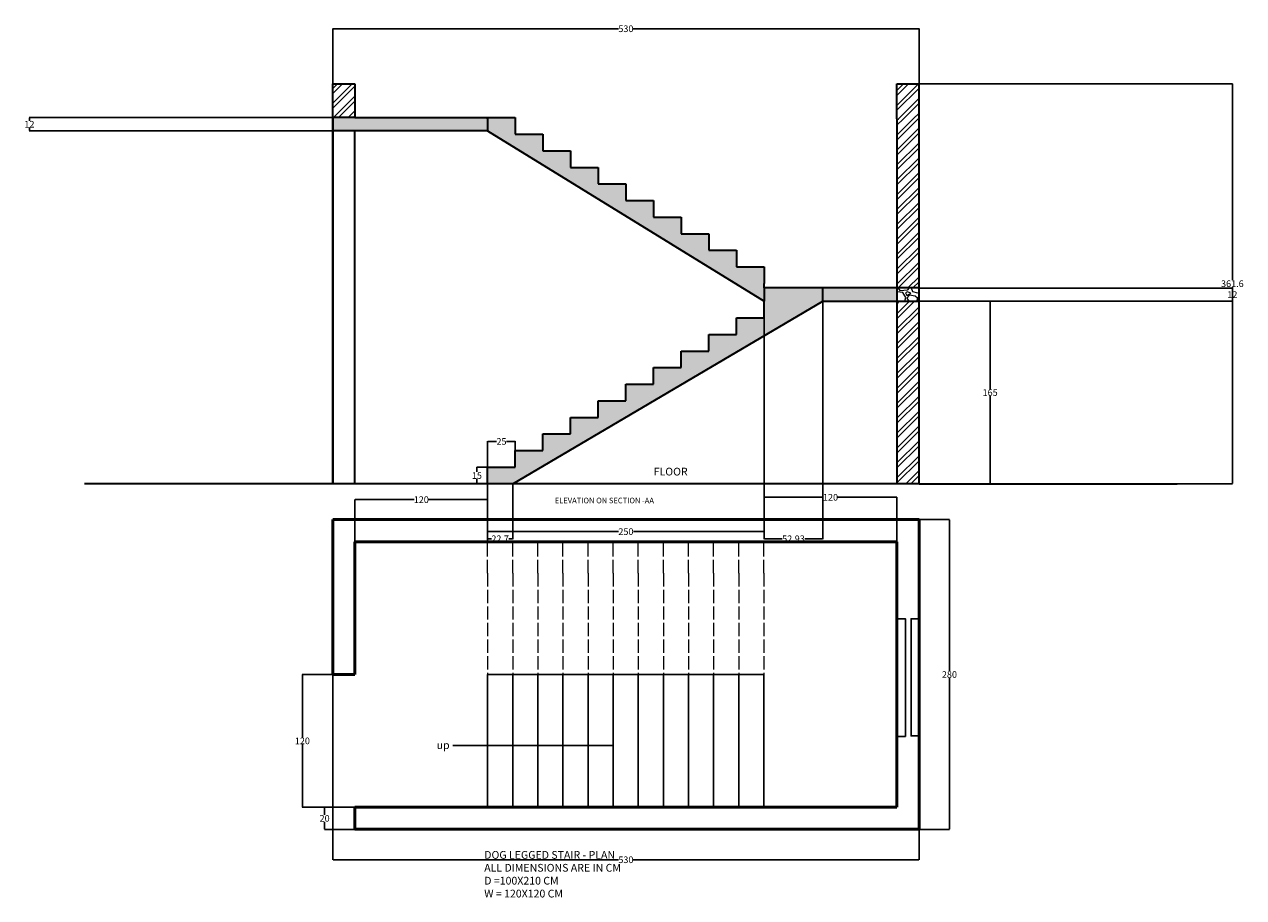
# Model space of a CAD drawing. Units: centimetres. Extents: x 1453 to 2556, y 1176 to 1965.
import ezdxf

# ---------------------------------------------------------------- set-up
doc = ezdxf.new("R2010")
doc.units = ezdxf.units.CM
doc.linetypes.add('ACAD_ISO02W100', pattern=[15, 12, -3])
for name, color, linetype, lineweight in [('A-ANNO-DIMS', 2, 'Continuous', 18), ('A-ANNO-TEXT', 7, 'Continuous', 18), ('A-FLOR-STRS', 3, 'Continuous', 25), ('A-FLOR-STRS-OVHD', 3, 'ACAD_ISO02W100', 18), ('A-GLAZ', 4, 'Continuous', 25), ('A-SECT', 1, 'Continuous', 35), ('A-WALL', 7, 'Continuous', 50), ('A-WALL-PATT', 8, 'Continuous', 18)]:
    doc.layers.add(name, color=color, linetype=linetype, lineweight=lineweight)
doc.styles.get("Standard").update_dxf_attribs({"font": 'arial.ttf'})
doc.dimstyles.get("Standard").update_dxf_attribs({"dimtxt": 6, "dimasz": 0.18, "dimexe": 0.18, "dimexo": 0.0625, "dimgap": 0.09, "dimtad": 0, "dimtih": 1, "dimtoh": 1, "dimdec": 0, "dimzin": 0, "dimdsep": 46, "dimtxsty": 'Standard', "dimcen": 0.09, "dimadec": 0, "dimazin": 0, "dimtfac": 1, "dimtdec": 0, "dimtofl": 0, "dimtmove": 0, "dimatfit": 3, "dimfxl": 1, "dimtolj": 1, "dimtzin": 0, "dimarcsym": 0})

# ---------------------------------------------------------------- blocks, each defined once
blk = doc.blocks.new('*D1')
at = {"layer": 'A-ANNO-DIMS', "color": 0, "lineweight": -2, "transparency": 16777216}
for p, q in [((1752.1, 1257.4), (1724.6, 1257.4)), ((1724.8, 1257.3), (1724.8, 1250.6)), ((1752.1, 1237.4), (1724.6, 1237.4)), ((1724.8, 1237.6), (1724.8, 1244.3))]:
    blk.add_line(p, q, dxfattribs=at)
at = {"layer": 'A-ANNO-DIMS', "color": 0, "transparency": 16777216}
for points in [[(1724.8, 1257.3), (1724.8, 1257.3), (1724.8, 1257.4)], [(1724.8, 1237.6), (1724.8, 1237.6), (1724.8, 1237.4)]]:
    blk.add_solid(points, dxfattribs=at)
at = {"layer": 'Defpoints', "color": 0, "transparency": 16777216}
for p in [(1752.2, 1257.4), (1724.8, 1237.4), (1752.2, 1237.4)]:
    blk.add_point(p, dxfattribs=at)
at = {"layer": 'A-ANNO-DIMS', "color": 0, "transparency": 16777216, "insert": (1724.8, 1247.4), "char_height": 6, "attachment_point": 5}
blk.add_mtext('\\A1;20', dxfattribs=at)
blk = doc.blocks.new('*D2')
at = {"layer": 'A-ANNO-DIMS', "color": 0, "lineweight": -2, "transparency": 16777216}
for p, q in [((1752.2, 1497.5), (1752.2, 1535.7)), ((1752.4, 1535.5), (1805.8, 1535.5)), ((1872, 1535.5), (1818.6, 1535.5)), ((1872.2, 1497.5), (1872.2, 1535.7))]:
    blk.add_line(p, q, dxfattribs=at)
at = {"layer": 'A-ANNO-DIMS', "color": 0, "transparency": 16777216}
for points in [[(1752.4, 1535.5), (1752.4, 1535.5), (1752.2, 1535.5)], [(1872, 1535.5), (1872, 1535.5), (1872.2, 1535.5)]]:
    blk.add_solid(points, dxfattribs=at)
at = {"layer": 'Defpoints', "color": 0, "transparency": 16777216}
for p in [(1752.2, 1535.5), (1752.2, 1497.4), (1872.2, 1497.4)]:
    blk.add_point(p, dxfattribs=at)
at = {"layer": 'A-ANNO-DIMS', "color": 0, "transparency": 16777216, "insert": (1812.2, 1535.5), "char_height": 6, "attachment_point": 5}
blk.add_mtext('\\A1;120', dxfattribs=at)
blk = doc.blocks.new('*D3')
at = {"layer": 'A-ANNO-DIMS', "color": 0, "lineweight": -2, "transparency": 16777216}
for p, q in [((1872.2, 1517.4), (1872.2, 1506.5)), ((2122.2, 1517.4), (2122.2, 1506.5)), ((1872.4, 1506.6), (1990.4, 1506.6)), ((2122, 1506.6), (2004, 1506.6))]:
    blk.add_line(p, q, dxfattribs=at)
at = {"layer": 'A-ANNO-DIMS', "color": 0, "transparency": 16777216}
for points in [[(1872.4, 1506.7), (1872.4, 1506.6), (1872.2, 1506.6)], [(2122, 1506.7), (2122, 1506.6), (2122.2, 1506.6)]]:
    blk.add_solid(points, dxfattribs=at)
at = {"layer": 'Defpoints', "color": 0, "transparency": 16777216}
for p in [(1872.2, 1517.4), (2122.2, 1517.4), (2122.2, 1506.6)]:
    blk.add_point(p, dxfattribs=at)
at = {"layer": 'A-ANNO-DIMS', "color": 0, "transparency": 16777216, "insert": (1997.2, 1506.6), "char_height": 6, "attachment_point": 5}
blk.add_mtext('\\A1;250', dxfattribs=at)
blk = doc.blocks.new('*D4')
at = {"layer": 'A-ANNO-DIMS', "color": 0, "lineweight": -2, "transparency": 16777216}
for p, q in [((2122.2, 1517.5), (2122.2, 1537.7)), ((2122.4, 1537.6), (2175.8, 1537.6)), ((2242, 1537.6), (2188.6, 1537.6)), ((2242.2, 1497.5), (2242.2, 1537.7))]:
    blk.add_line(p, q, dxfattribs=at)
at = {"layer": 'A-ANNO-DIMS', "color": 0, "transparency": 16777216}
for points in [[(2122.4, 1537.6), (2122.4, 1537.5), (2122.2, 1537.6)], [(2242, 1537.6), (2242, 1537.5), (2242.2, 1537.6)]]:
    blk.add_solid(points, dxfattribs=at)
at = {"layer": 'Defpoints', "color": 0, "transparency": 16777216}
for p in [(2242.2, 1537.6), (2122.2, 1517.4), (2242.2, 1497.4)]:
    blk.add_point(p, dxfattribs=at)
at = {"layer": 'A-ANNO-DIMS', "color": 0, "transparency": 16777216, "insert": (2182.2, 1537.6), "char_height": 6, "attachment_point": 5}
blk.add_mtext('\\A1;120', dxfattribs=at)
blk = doc.blocks.new('*D5')
at = {"layer": 'A-ANNO-DIMS', "color": 0, "lineweight": -2, "transparency": 16777216}
for p, q in [((1872.1, 1564.8), (1862.3, 1564.8)), ((1862.5, 1564.7), (1862.5, 1560.5)), ((1872.1, 1549.8), (1862.3, 1549.8)), ((1862.5, 1550), (1862.5, 1554.2))]:
    blk.add_line(p, q, dxfattribs=at)
at = {"layer": 'A-ANNO-DIMS', "color": 0, "transparency": 16777216}
for points in [[(1862.5, 1564.7), (1862.5, 1564.7), (1862.5, 1564.8)], [(1862.5, 1550), (1862.5, 1550), (1862.5, 1549.8)]]:
    blk.add_solid(points, dxfattribs=at)
at = {"layer": 'Defpoints', "color": 0, "transparency": 16777216}
for p in [(1862.5, 1564.8), (1872.2, 1564.8), (1872.2, 1549.8)]:
    blk.add_point(p, dxfattribs=at)
at = {"layer": 'A-ANNO-DIMS', "color": 0, "transparency": 16777216, "insert": (1862.5, 1557.3), "char_height": 6, "attachment_point": 5}
blk.add_mtext('\\A1;15', dxfattribs=at)
blk = doc.blocks.new('*D6')
at = {"layer": 'A-ANNO-DIMS', "color": 0, "lineweight": -2, "transparency": 16777216}
for p, q in [((1872.2, 1564.9), (1872.2, 1588.3)), ((1872.4, 1588.1), (1880.2, 1588.1)), ((1897, 1588.1), (1889.2, 1588.1)), ((1897.2, 1564.9), (1897.2, 1588.3))]:
    blk.add_line(p, q, dxfattribs=at)
at = {"layer": 'A-ANNO-DIMS', "color": 0, "transparency": 16777216}
for points in [[(1872.4, 1588.2), (1872.4, 1588.1), (1872.2, 1588.1)], [(1897, 1588.2), (1897, 1588.1), (1897.2, 1588.1)]]:
    blk.add_solid(points, dxfattribs=at)
at = {"layer": 'Defpoints', "color": 0, "transparency": 16777216}
for p in [(1897.2, 1588.1), (1872.2, 1564.8), (1897.2, 1564.8)]:
    blk.add_point(p, dxfattribs=at)
at = {"layer": 'A-ANNO-DIMS', "color": 0, "transparency": 16777216, "insert": (1884.7, 1588.1), "char_height": 6, "attachment_point": 5}
blk.add_mtext('\\A1;25', dxfattribs=at)
blk = doc.blocks.new('*D7')
at = {"layer": 'A-ANNO-DIMS', "color": 0, "lineweight": -2, "transparency": 16777216}
for p, q in [((2262.3, 1714.8), (2326.7, 1714.8)), ((2326.5, 1714.7), (2326.5, 1635.5)), ((2326.5, 1550), (2326.5, 1629.2)), ((2262.3, 1549.8), (2326.7, 1549.8))]:
    blk.add_line(p, q, dxfattribs=at)
at = {"layer": 'A-ANNO-DIMS', "color": 0, "transparency": 16777216}
for points in [[(2326.5, 1714.7), (2326.6, 1714.7), (2326.5, 1714.8)], [(2326.5, 1550), (2326.6, 1550), (2326.5, 1549.8)]]:
    blk.add_solid(points, dxfattribs=at)
at = {"layer": 'Defpoints', "color": 0, "transparency": 16777216}
for p in [(2262.2, 1714.8), (2326.5, 1714.8), (2262.2, 1549.8)]:
    blk.add_point(p, dxfattribs=at)
at = {"layer": 'A-ANNO-DIMS', "color": 0, "transparency": 16777216, "insert": (2326.5, 1632.3), "char_height": 6, "attachment_point": 5}
blk.add_mtext('\\A1;165', dxfattribs=at)
blk = doc.blocks.new('*D8')
at = {"layer": 'A-ANNO-DIMS', "color": 0, "lineweight": -2, "transparency": 16777216}
for p, q in [((1732.2, 1377.4), (1732.2, 1209.8)), ((2262.2, 1237.4), (2262.2, 1209.8)), ((1732.4, 1209.9), (1990.5, 1209.9)), ((2262, 1209.9), (2003.9, 1209.9))]:
    blk.add_line(p, q, dxfattribs=at)
at = {"layer": 'A-ANNO-DIMS', "color": 0, "transparency": 16777216}
for points in [[(1732.4, 1210), (1732.4, 1209.9), (1732.2, 1209.9)], [(2262, 1210), (2262, 1209.9), (2262.2, 1209.9)]]:
    blk.add_solid(points, dxfattribs=at)
at = {"layer": 'Defpoints', "color": 0, "transparency": 16777216}
for p in [(1732.2, 1377.4), (2262.2, 1237.4), (2262.2, 1209.9)]:
    blk.add_point(p, dxfattribs=at)
at = {"layer": 'A-ANNO-DIMS', "color": 0, "transparency": 16777216, "insert": (1997.2, 1209.9), "char_height": 6, "attachment_point": 5}
blk.add_mtext('\\A1;530', dxfattribs=at)
blk = doc.blocks.new('*D9')
at = {"layer": 'A-ANNO-DIMS', "color": 0, "lineweight": -2, "transparency": 16777216}
for p, q in [((2262.3, 1517.4), (2289.9, 1517.4)), ((2289.7, 1517.3), (2289.7, 1380.6)), ((2289.7, 1237.6), (2289.7, 1374.3)), ((2262.3, 1237.4), (2289.9, 1237.4))]:
    blk.add_line(p, q, dxfattribs=at)
at = {"layer": 'A-ANNO-DIMS', "color": 0, "transparency": 16777216}
for points in [[(2289.7, 1517.3), (2289.7, 1517.3), (2289.7, 1517.4)], [(2289.7, 1237.6), (2289.7, 1237.6), (2289.7, 1237.4)]]:
    blk.add_solid(points, dxfattribs=at)
at = {"layer": 'Defpoints', "color": 0, "transparency": 16777216}
for p in [(2262.2, 1517.4), (2289.7, 1517.4), (2262.2, 1237.4)]:
    blk.add_point(p, dxfattribs=at)
at = {"layer": 'A-ANNO-DIMS', "color": 0, "transparency": 16777216, "insert": (2289.7, 1377.4), "char_height": 6, "attachment_point": 5}
blk.add_mtext('\\A1;280', dxfattribs=at)
blk = doc.blocks.new('*D10')
at = {"layer": 'A-ANNO-DIMS', "color": 0, "lineweight": -2, "transparency": 16777216}
for p, q in [((1752.1, 1377.4), (1704.5, 1377.4)), ((1704.7, 1377.3), (1704.7, 1320.6)), ((1704.7, 1257.6), (1704.7, 1314.3)), ((1752.1, 1257.4), (1704.5, 1257.4))]:
    blk.add_line(p, q, dxfattribs=at)
at = {"layer": 'A-ANNO-DIMS', "color": 0, "transparency": 16777216}
for points in [[(1704.7, 1377.3), (1704.7, 1377.3), (1704.7, 1377.4)], [(1704.7, 1257.6), (1704.7, 1257.6), (1704.7, 1257.4)]]:
    blk.add_solid(points, dxfattribs=at)
at = {"layer": 'Defpoints', "color": 0, "transparency": 16777216}
for p in [(1704.7, 1377.4), (1752.2, 1377.4), (1752.2, 1257.4)]:
    blk.add_point(p, dxfattribs=at)
at = {"layer": 'A-ANNO-DIMS', "color": 0, "transparency": 16777216, "insert": (1704.7, 1317.4), "char_height": 6, "attachment_point": 5}
blk.add_mtext('\\A1;120', dxfattribs=at)
blk = doc.blocks.new('*D11')
at = {"layer": 'A-ANNO-DIMS', "color": 0, "lineweight": -2, "transparency": 16777216}
for p, q in [((2262.3, 1911.5), (2545.6, 1911.5)), ((2545.5, 1911.3), (2545.5, 1733.8)), ((2545.5, 1550), (2545.5, 1727.5)), ((2262.3, 1549.8), (2545.6, 1549.8))]:
    blk.add_line(p, q, dxfattribs=at)
at = {"layer": 'A-ANNO-DIMS', "color": 0, "transparency": 16777216}
for points in [[(2545.4, 1911.3), (2545.5, 1911.3), (2545.5, 1911.5)], [(2545.4, 1550), (2545.5, 1550), (2545.5, 1549.8)]]:
    blk.add_solid(points, dxfattribs=at)
at = {"layer": 'Defpoints', "color": 0, "transparency": 16777216}
for p in [(2262.2, 1911.5), (2545.5, 1911.5), (2262.2, 1549.8)]:
    blk.add_point(p, dxfattribs=at)
at = {"layer": 'A-ANNO-DIMS', "color": 0, "transparency": 16777216, "insert": (2545.5, 1730.7), "char_height": 6, "attachment_point": 5}
blk.add_mtext('\\A1;361.6', dxfattribs=at)
blk = doc.blocks.new('*D12')
at = {"layer": 'A-ANNO-DIMS', "color": 0, "lineweight": -2, "transparency": 16777216}
for p, q in [((1732.2, 1911.5), (1732.2, 1961.4)), ((1732.4, 1961.2), (1990.5, 1961.2)), ((2262, 1961.2), (2003.9, 1961.2)), ((2262.2, 1911.5), (2262.2, 1961.4))]:
    blk.add_line(p, q, dxfattribs=at)
at = {"layer": 'A-ANNO-DIMS', "color": 0, "transparency": 16777216}
for points in [[(1732.4, 1961.2), (1732.4, 1961.2), (1732.2, 1961.2)], [(2262, 1961.2), (2262, 1961.2), (2262.2, 1961.2)]]:
    blk.add_solid(points, dxfattribs=at)
at = {"layer": 'Defpoints', "color": 0, "transparency": 16777216}
for p in [(2262.2, 1961.2), (1732.2, 1911.5), (2262.2, 1911.5)]:
    blk.add_point(p, dxfattribs=at)
at = {"layer": 'A-ANNO-DIMS', "color": 0, "transparency": 16777216, "insert": (1997.2, 1961.2), "char_height": 6, "attachment_point": 5}
blk.add_mtext('\\A1;530', dxfattribs=at)
blk = doc.blocks.new('*D13')
at = {"layer": 'A-ANNO-DIMS', "color": 0, "lineweight": -2, "transparency": 16777216}
for p, q in [((1752.1, 1880.9), (1457.7, 1880.9)), ((1457.9, 1880.7), (1457.9, 1878)), ((1752.1, 1868.9), (1457.7, 1868.9)), ((1457.9, 1869.1), (1457.9, 1871.8))]:
    blk.add_line(p, q, dxfattribs=at)
at = {"layer": 'A-ANNO-DIMS', "color": 0, "transparency": 16777216}
for points in [[(1457.9, 1880.7), (1457.9, 1880.7), (1457.9, 1880.9)], [(1457.9, 1869.1), (1457.9, 1869.1), (1457.9, 1868.9)]]:
    blk.add_solid(points, dxfattribs=at)
at = {"layer": 'Defpoints', "color": 0, "transparency": 16777216}
for p in [(1752.2, 1880.9), (1457.9, 1868.9), (1752.2, 1868.9)]:
    blk.add_point(p, dxfattribs=at)
at = {"layer": 'A-ANNO-DIMS', "color": 0, "transparency": 16777216, "insert": (1457.9, 1874.9), "char_height": 6, "attachment_point": 5}
blk.add_mtext('\\A1;12', dxfattribs=at)
blk = doc.blocks.new('*D14')
at = {"layer": 'A-ANNO-DIMS', "color": 0, "lineweight": -2, "transparency": 16777216}
for p, q in [((2262.3, 1726.8), (2545.6, 1726.8)), ((2545.5, 1726.7), (2545.5, 1723.9)), ((2262.3, 1714.8), (2545.6, 1714.8)), ((2545.5, 1715), (2545.5, 1717.7))]:
    blk.add_line(p, q, dxfattribs=at)
at = {"layer": 'A-ANNO-DIMS', "color": 0, "transparency": 16777216}
for points in [[(2545.4, 1726.7), (2545.5, 1726.7), (2545.5, 1726.8)], [(2545.4, 1715), (2545.5, 1715), (2545.5, 1714.8)]]:
    blk.add_solid(points, dxfattribs=at)
at = {"layer": 'Defpoints', "color": 0, "transparency": 16777216}
for p in [(2262.2, 1726.8), (2262.2, 1714.8), (2545.5, 1714.8)]:
    blk.add_point(p, dxfattribs=at)
at = {"layer": 'A-ANNO-DIMS', "color": 0, "transparency": 16777216, "insert": (2545.5, 1720.8), "char_height": 6, "attachment_point": 5}
blk.add_mtext('\\A1;12', dxfattribs=at)
blk = doc.blocks.new('*D15')
at = {"layer": 'A-ANNO-DIMS', "color": 0, "lineweight": -2, "transparency": 16777216}
for p, q in [((1872.2, 1549.8), (1872.2, 1499.9)), ((1894.9, 1549.8), (1894.9, 1499.9)), ((1872.4, 1500.1), (1875.6, 1500.1)), ((1894.7, 1500.1), (1891.5, 1500.1))]:
    blk.add_line(p, q, dxfattribs=at)
at = {"layer": 'A-ANNO-DIMS', "color": 0, "transparency": 16777216}
for points in [[(1872.4, 1500.1), (1872.4, 1500.1), (1872.2, 1500.1)], [(1894.7, 1500.1), (1894.7, 1500.1), (1894.9, 1500.1)]]:
    blk.add_solid(points, dxfattribs=at)
at = {"layer": 'Defpoints', "color": 0, "transparency": 16777216}
for p in [(1872.2, 1549.8), (1894.9, 1549.8), (1894.9, 1500.1)]:
    blk.add_point(p, dxfattribs=at)
at = {"layer": 'A-ANNO-DIMS', "color": 0, "transparency": 16777216, "insert": (1883.5, 1500.1), "char_height": 6, "attachment_point": 5}
blk.add_mtext('\\A1;22.7', dxfattribs=at)
blk = doc.blocks.new('*D16')
at = {"layer": 'A-ANNO-DIMS', "color": 0, "lineweight": -2, "transparency": 16777216}
for p, q in [((2122.2, 1714.8), (2122.2, 1499.9)), ((2175.1, 1714.8), (2175.1, 1499.9)), ((2122.4, 1500.1), (2138.4, 1500.1)), ((2174.9, 1500.1), (2158.9, 1500.1))]:
    blk.add_line(p, q, dxfattribs=at)
at = {"layer": 'A-ANNO-DIMS', "color": 0, "transparency": 16777216}
for points in [[(2122.4, 1500.1), (2122.4, 1500.1), (2122.2, 1500.1)], [(2174.9, 1500.1), (2174.9, 1500.1), (2175.1, 1500.1)]]:
    blk.add_solid(points, dxfattribs=at)
at = {"layer": 'Defpoints', "color": 0, "transparency": 16777216}
for p in [(2122.2, 1714.8), (2175.1, 1714.8), (2175.1, 1500.1)]:
    blk.add_point(p, dxfattribs=at)
at = {"layer": 'A-ANNO-DIMS', "color": 0, "transparency": 16777216, "insert": (2148.7, 1500.1), "char_height": 6, "attachment_point": 5}
blk.add_mtext('\\A1;52.93', dxfattribs=at)

msp = doc.modelspace()

# ---------------------------------------------------------------- hatches: boundary and pattern name
at = {"layer": 'A-WALL-PATT'}
h = msp.add_hatch(dxfattribs=at)
h.set_pattern_fill('ANSI32', color=256)
h.paths.add_polyline_path([(2262.194, 1879.847), (2242.194, 1879.847), (2242.194, 1726.847), (2262.194, 1726.847), (2262.194, 1734.847)])
h.paths.add_polyline_path([(2262.194, 1714.847), (2242.194, 1714.847), (2242.194, 1549.847), (2262.194, 1549.847)])
h.paths.add_polyline_path([(1752.194, 1911.468), (1732.194, 1911.468), (1732.194, 1880.917), (1752.194, 1880.917)])
h = msp.add_hatch(dxfattribs=at)
h.set_pattern_fill('ANSI32', color=256)
h.paths.add_polyline_path([(2262.194, 1911.468), (2242.194, 1911.468), (2242.194, 1879.847), (2262.194, 1879.847)])
h = msp.add_hatch(dxfattribs=at)
h.set_pattern_fill('GRAVEL', color=256)
h.paths.add_polyline_path([(1997.194, 1820.917), (1972.194, 1820.917), (1972.194, 1835.917), (1947.194, 1835.917), (1947.194, 1850.917), (1922.194, 1850.917), (1922.194, 1865.917), (1897.194, 1865.917), (1897.194, 1880.917), (1872.194, 1880.917), (1872.194, 1868.917), (2122.194, 1714.847), (2122.194, 1726.847), (2122.194, 1730.917), (2122.194, 1745.917), (2097.194, 1745.917), (2097.194, 1760.917), (2072.194, 1760.917), (2072.194, 1775.917), (2047.194, 1775.917), (2047.194, 1790.917), (2022.194, 1790.917), (2022.194, 1805.917), (1997.194, 1805.917)])
h.paths.add_polyline_path([(2175.123, 1714.847), (2175.123, 1726.847), (2122.194, 1726.847), (2122.194, 1714.847), (2122.194, 1699.847), (2097.194, 1699.847), (2097.194, 1684.847), (2072.194, 1684.847), (2072.194, 1669.847), (2047.194, 1669.847), (2047.194, 1654.847), (2022.194, 1654.847), (2022.194, 1639.847), (1997.194, 1639.847), (1997.194, 1624.847), (1972.194, 1624.847), (1972.194, 1609.847), (1947.194, 1609.847), (1947.194, 1594.847), (1922.194, 1594.847), (1922.194, 1579.847), (1897.194, 1579.847), (1897.194, 1564.847), (1872.194, 1564.847), (1872.194, 1549.847), (1894.894, 1549.847)])
h.paths.add_polyline_path([(2242.194, 1726.847), (2175.123, 1726.847), (2175.123, 1714.847), (2242.194, 1714.847)])
h.paths.add_polyline_path([(1872.194, 1880.917), (1752.194, 1880.917), (1732.194, 1880.917), (1732.194, 1868.917), (1872.194, 1868.917)])
h = msp.add_hatch(dxfattribs=at)
h.set_pattern_fill('GRAVEL', color=256)
h.paths.add_polyline_path([(2262.194, 1726.847), (2242.194, 1726.847), (2242.194, 1714.847), (2262.194, 1714.847)])

# ---------------------------------------------------------------- linework, layer by layer
at = {"layer": 'A-FLOR-STRS'}
for p, q in [((1872.194, 1377.43), (1872.194, 1257.43)), ((2121.894, 1377.43), (1872.194, 1377.43)), ((1894.894, 1377.43), (1894.894, 1257.43)), ((1917.594, 1377.43), (1917.594, 1257.43)), ((1940.294, 1377.43), (1940.294, 1257.43)), ((1962.994, 1377.43), (1962.994, 1257.43)), ((1985.694, 1377.43), (1985.694, 1257.43)), ((2008.394, 1377.43), (2008.394, 1257.43)), ((2031.094, 1377.43), (2031.094, 1257.43)), ((2053.794, 1377.43), (2053.794, 1257.43)), ((2076.494, 1377.43), (2076.494, 1257.43)), ((2099.194, 1377.43), (2099.194, 1257.43)), ((2121.894, 1377.43), (2121.894, 1257.43)), ((1840.674, 1313.105), (1985.694, 1313.105))]:
    msp.add_line(p, q, dxfattribs=at)
at = {"layer": 'A-FLOR-STRS-OVHD'}
for p, q in [((1872.194, 1468.986), (1872.194, 1497.43)), ((1894.894, 1468.986), (1894.894, 1497.43)), ((1917.594, 1468.986), (1917.594, 1497.43)), ((1940.294, 1468.986), (1940.294, 1497.43)), ((1962.994, 1468.986), (1962.994, 1497.43)), ((1985.694, 1468.986), (1985.694, 1497.43)), ((2008.394, 1468.986), (2008.394, 1497.43)), ((2031.094, 1468.986), (2031.094, 1497.43)), ((2053.794, 1468.986), (2053.794, 1497.43)), ((2076.494, 1468.986), (2076.494, 1497.43)), ((2099.194, 1468.986), (2099.194, 1497.43)), ((2121.894, 1468.986), (2121.894, 1497.43)), ((1872.194, 1468.986), (1872.194, 1377.43)), ((1894.894, 1468.986), (1894.894, 1377.43)), ((1917.594, 1468.986), (1917.594, 1377.43)), ((1940.294, 1468.986), (1940.294, 1377.43)), ((1962.994, 1468.986), (1962.994, 1377.43)), ((1985.694, 1468.986), (1985.694, 1377.43)), ((2008.394, 1468.986), (2008.394, 1377.43)), ((2031.094, 1468.986), (2031.094, 1377.43)), ((2053.794, 1468.986), (2053.794, 1377.43)), ((2076.494, 1468.986), (2076.494, 1377.43)), ((2099.194, 1468.986), (2099.194, 1377.43)), ((2121.894, 1468.986), (2121.894, 1377.43))]:
    msp.add_line(p, q, dxfattribs=at)
at = {"layer": 'A-GLAZ'}
for points in [[(2242.194, 1321.479), (2249.946, 1321.479), (2249.946, 1427.742), (2242.194, 1427.742)], [(2262.194, 1427.742), (2255, 1427.742), (2255, 1321.844), (2262.194, 1321.844)]]:
    msp.add_lwpolyline(points, dxfattribs=at)
at = {"layer": 'A-SECT'}
for p, q in [((1732.194, 1880.917), (1732.194, 1911.468)), ((1732.194, 1911.468), (1752.194, 1911.468)), ((1752.194, 1911.468), (1752.194, 1880.917)), ((2242.194, 1911.468), (2262.194, 1911.468)), ((2242.194, 1879.847), (2242.194, 1911.468)), ((2262.194, 1879.847), (2262.194, 1911.468)), ((1732.194, 1715.917), (1732.194, 1880.917)), ((1752.194, 1880.917), (1732.194, 1880.917)), ((1752.194, 1880.917), (1732.194, 1880.917)), ((1732.194, 1880.917), (1732.194, 1549.847)), ((1752.194, 1880.917), (1872.194, 1880.917)), ((1872.194, 1879.847), (1872.194, 1880.917)), ((1872.194, 1880.917), (1872.194, 1868.917)), ((1872.194, 1880.917), (1872.194, 1868.917)), ((1872.194, 1880.917), (1897.194, 1880.917)), ((1897.194, 1880.917), (1897.194, 1865.917)), ((2242.194, 1879.847), (2242.194, 1549.847)), ((2262.194, 1549.847), (2262.194, 1879.847)), ((1872.194, 1868.917), (1732.194, 1868.917)), ((1752.194, 1860.917), (1752.194, 1868.917)), ((1872.194, 1868.917), (2122.194, 1714.847)), ((1897.194, 1865.917), (1922.194, 1865.917)), ((1922.194, 1865.917), (1922.194, 1850.917)), ((1752.194, 1715.917), (1752.194, 1860.917)), ((1752.194, 1715.917), (1752.194, 1860.917)), ((1922.194, 1850.917), (1947.194, 1850.917)), ((1947.194, 1850.917), (1947.194, 1835.917)), ((1947.194, 1835.917), (1972.194, 1835.917)), ((1972.194, 1835.917), (1972.194, 1820.917)), ((1972.194, 1820.917), (1997.194, 1820.917)), ((1997.194, 1820.917), (1997.194, 1805.917)), ((1997.194, 1805.917), (2022.194, 1805.917)), ((2022.194, 1805.917), (2022.194, 1790.917)), ((2022.194, 1790.917), (2047.194, 1790.917)), ((2047.194, 1790.917), (2047.194, 1775.917)), ((2047.194, 1775.917), (2072.194, 1775.917)), ((2072.194, 1775.917), (2072.194, 1760.917)), ((2072.194, 1760.917), (2097.194, 1760.917)), ((2097.194, 1760.917), (2097.194, 1745.917)), ((2097.194, 1745.917), (2122.194, 1745.917)), ((2122.194, 1745.917), (2122.194, 1730.917)), ((2122.194, 1726.847), (2122.194, 1730.917)), ((2262.194, 1714.847), (2262.194, 1734.847)), ((2262.194, 1726.847), (2122.194, 1726.847)), ((2122.194, 1726.847), (2122.194, 1714.847)), ((2175.123, 1714.847), (2175.123, 1726.847)), ((2262.194, 1714.847), (2262.194, 1726.847)), ((1732.194, 1550.917), (1732.194, 1715.917)), ((1752.194, 1550.917), (1752.194, 1715.917)), ((1752.194, 1550.917), (1752.194, 1715.917)), ((1894.894, 1549.847), (2175.123, 1714.847)), ((2122.194, 1699.847), (2122.194, 1714.847)), ((2175.123, 1714.847), (2262.194, 1714.847)), ((2262.194, 1549.847), (2262.194, 1714.847)), ((2097.194, 1684.847), (2097.194, 1699.847)), ((2097.194, 1699.847), (2122.194, 1699.847)), ((2072.194, 1669.847), (2072.194, 1684.847)), ((2072.194, 1684.847), (2097.194, 1684.847)), ((2047.194, 1654.847), (2047.194, 1669.847)), ((2047.194, 1669.847), (2072.194, 1669.847)), ((2022.194, 1639.847), (2022.194, 1654.847)), ((2022.194, 1654.847), (2047.194, 1654.847)), ((1997.194, 1624.847), (1997.194, 1639.847)), ((1997.194, 1639.847), (2022.194, 1639.847)), ((1972.194, 1609.847), (1972.194, 1624.847)), ((1972.194, 1624.847), (1997.194, 1624.847)), ((1947.194, 1594.847), (1947.194, 1609.847)), ((1947.194, 1609.847), (1972.194, 1609.847)), ((1922.194, 1579.847), (1922.194, 1594.847)), ((1922.194, 1594.847), (1947.194, 1594.847)), ((1897.194, 1564.847), (1897.194, 1579.847)), ((1897.194, 1579.847), (1922.194, 1579.847)), ((1872.194, 1549.847), (1872.194, 1564.847)), ((1872.194, 1564.847), (1897.194, 1564.847)), ((2262.194, 1549.847), (1507.652, 1549.847)), ((1732.194, 1550.917), (1732.194, 1549.847)), ((2262.194, 1549.847), (2391.916, 1549.847)), ((2391.916, 1549.847), (2495.702, 1549.847))]:
    msp.add_line(p, q, dxfattribs=at)
at = {"layer": 'A-WALL'}
for p, q in [((1732.194, 1377.43), (1732.194, 1517.43)), ((1752.194, 1517.43), (1732.194, 1517.43)), ((1752.194, 1517.43), (1872.194, 1517.43)), ((1872.194, 1517.43), (2122.194, 1517.43)), ((2122.194, 1517.43), (2262.194, 1517.43)), ((2262.194, 1517.43), (2262.194, 1237.43)), ((1752.194, 1497.43), (1872.194, 1497.43)), ((1752.194, 1497.43), (1752.194, 1377.43)), ((1872.194, 1497.43), (2122.194, 1497.43)), ((2122.194, 1497.43), (2242.194, 1497.43)), ((2242.194, 1497.43), (2242.194, 1257.43)), ((2242.194, 1497.43), (2242.194, 1377.43)), ((1752.194, 1377.43), (1732.194, 1377.43)), ((2242.194, 1257.43), (1752.194, 1257.43)), ((1752.194, 1257.43), (1752.194, 1237.43)), ((2262.194, 1237.43), (1752.194, 1237.43))]:
    msp.add_line(p, q, dxfattribs=at)

# ---------------------------------------------------------------- texts
at = {"layer": 'A-ANNO-TEXT', "attachment_point": 1}
for s, width, insert, char_height in [('{\\fArial|b1|i0|c0|p34;FLOOR}', 182.85356, (2022.331, 1564.333), 7), ('{\\fArial|b1|i0|c0|p34;ELEVATION ON SECTION -AA}', 204.81193, (1932.901, 1537.206), 5), ('{\\fArial|b1|i0|c0|p34;up}', 24.40783, (1826.108, 1317.038), 7), ('{\\fArial|b1|i0|c0|p34;DOG LEGGED STAIR - PLAN\\PALL DIMENSIONS ARE IN CM\\PD =100X210 CM\\PW = 120X120 CM}', 252.59856, (1869.112, 1217.826), 7)]:
    msp.add_mtext_dynamic_manual_height_columns(s, width=width, gutter_width=12.5, heights=[0], dxfattribs=dict(at, insert=insert, char_height=char_height))

# ---------------------------------------------------------------- dimensions: what is measured, and where the dimension line sits
at = {"layer": 'A-ANNO-DIMS'}
for base, p1, p2, override, picture, middle in [((2262.194, 1961.218), (1732.194, 1911.468), (2262.194, 1911.468), {"dimdec": 0, "dimlfac": 1, "dimrnd": 0, "dimzin": 0, "dimdsep": 46, "dimlunit": 2}, '*D12', (1997.194, 1961.218)), ((2175.123, 1500.097), (2122.194, 1714.847), (2175.123, 1714.847), {"dimdec": 2, "dimlfac": 1, "dimrnd": 0, "dimzin": 0, "dimdsep": 46, "dimlunit": 2}, '*D16', (2148.658, 1500.097)), ((1897.194, 1588.124), (1872.194, 1564.847), (1897.194, 1564.847), {"dimclrd": 0, "dimclre": 0, "dimclrt": 0}, '*D6', (1884.694, 1588.124)), ((1894.894, 1500.097), (1872.194, 1549.847), (1894.894, 1549.847), {"dimdec": 1, "dimlfac": 1, "dimrnd": 0, "dimzin": 0, "dimdsep": 46, "dimlunit": 2}, '*D15', (1883.544, 1500.097)), ((1752.194, 1535.484), (1872.194, 1497.43), (1752.194, 1497.43), {"dimclrd": 0, "dimclre": 0, "dimclrt": 0}, '*D2', (1812.194, 1535.484)), ((2242.194, 1537.558), (2122.194, 1517.43), (2242.194, 1497.43), {"dimclrd": 0, "dimclre": 0, "dimclrt": 0}, '*D4', (2182.194, 1537.558)), ((2122.194, 1506.646), (1872.194, 1517.43), (2122.194, 1517.43), {"dimclrd": 0, "dimclre": 0, "dimclrt": 0}, '*D3', (1997.194, 1506.646)), ((2262.194, 1209.93), (1732.194, 1377.43), (2262.194, 1237.43), {"dimdec": 0, "dimlfac": 1, "dimrnd": 0, "dimzin": 0, "dimdsep": 46, "dimlunit": 2}, '*D8', (1997.194, 1209.93))]:
    dim = msp.add_linear_dim(base=base, p1=p1, p2=p2, dimstyle='Standard', override=override, dxfattribs=at)
    dim.commit()
    dim.dimension.update_dxf_attribs({"geometry": picture, "text_midpoint": middle})
for base, p1, p2, override, picture, middle in [((2545.452, 1911.468), (2262.194, 1549.847), (2262.194, 1911.468), {"dimdec": 1, "dimlfac": 1, "dimrnd": 0, "dimzin": 0, "dimdsep": 46, "dimlunit": 2}, '*D11', (2545.452, 1730.657)), ((1457.902, 1868.917), (1752.194, 1880.917), (1752.194, 1868.917), {"dimdec": 0, "dimlfac": 1, "dimrnd": 0, "dimzin": 0, "dimdsep": 46, "dimlunit": 2}, '*D13', (1457.902, 1874.917)), ((2545.452, 1714.847), (2262.194, 1726.847), (2262.194, 1714.847), {"dimdec": 0, "dimlfac": 1, "dimrnd": 0, "dimzin": 0, "dimdsep": 46, "dimlunit": 2}, '*D14', (2545.452, 1720.847)), ((2326.549, 1714.847), (2262.194, 1549.847), (2262.194, 1714.847), {"dimclrd": 0, "dimclre": 0, "dimclrt": 0}, '*D7', (2326.549, 1632.347)), ((1862.496, 1564.847), (1872.194, 1549.847), (1872.194, 1564.847), {"dimclrd": 0, "dimclre": 0, "dimclrt": 0}, '*D5', (1862.496, 1557.347)), ((2289.694, 1517.43), (2262.194, 1237.43), (2262.194, 1517.43), {"dimdec": 0, "dimlfac": 1, "dimrnd": 0, "dimzin": 0, "dimdsep": 46, "dimlunit": 2}, '*D9', (2289.694, 1377.43)), ((1704.694, 1377.43), (1752.194, 1257.43), (1752.194, 1377.43), {"dimdec": 0, "dimlfac": 1, "dimrnd": 0, "dimzin": 0, "dimdsep": 46, "dimlunit": 2}, '*D10', (1704.694, 1317.43)), ((1724.788, 1237.43), (1752.194, 1257.43), (1752.194, 1237.43), {"dimclrd": 0, "dimclre": 0, "dimclrt": 0}, '*D1', (1724.788, 1247.43))]:
    dim = msp.add_linear_dim(base=base, p1=p1, p2=p2, angle=90, dimstyle='Standard', override=override, dxfattribs=at)
    dim.commit()
    dim.dimension.update_dxf_attribs({"geometry": picture, "text_midpoint": middle})

doc.saveas('drawing.dxf')
